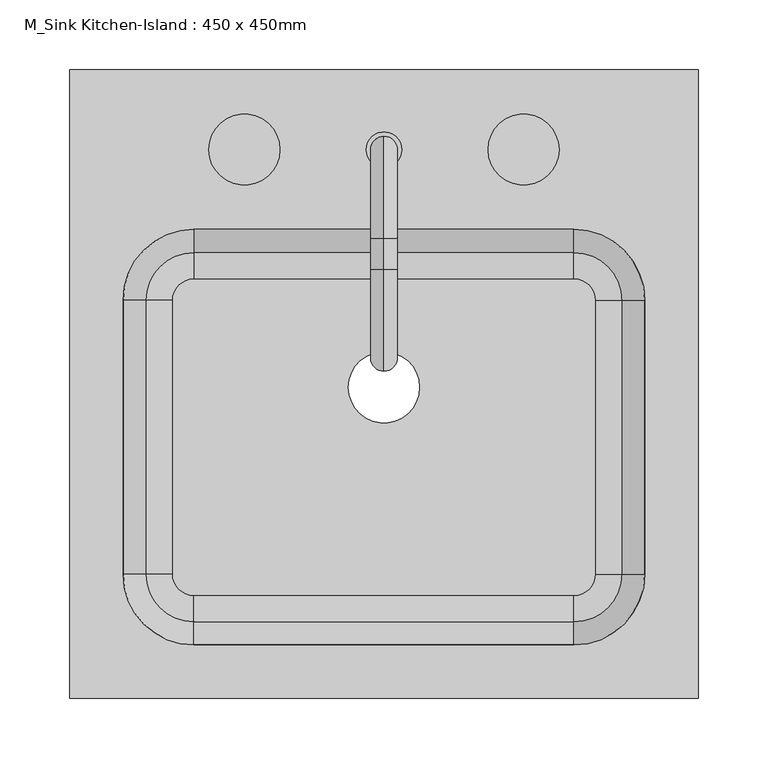
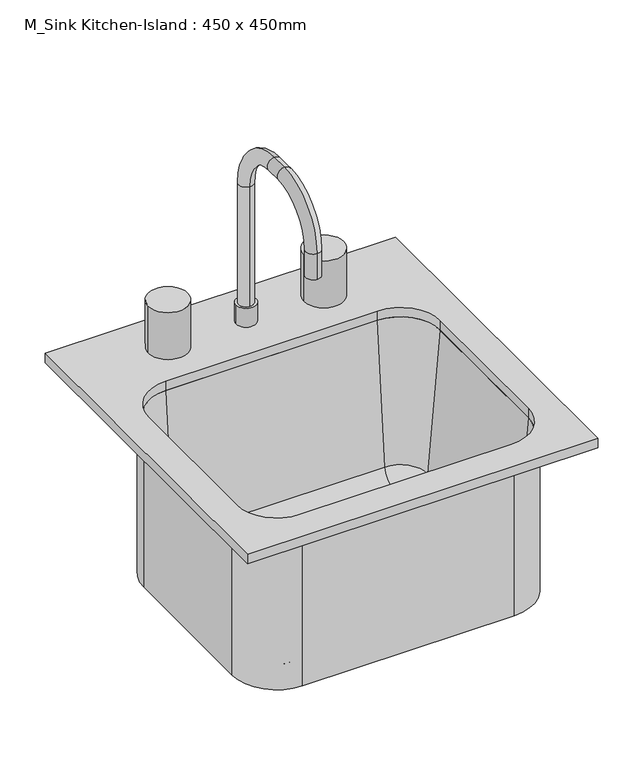
"""IFC4 building model written with IfcOpenShell, lengths in millimetres: flow terminal geometry, M_Sink Kitchen-Island : 450 x 450mm."""

from ifc_helpers import new_model, si_unit, point, frame, frame_2d, origin, place, context, project, spatial, polyline, circle_curve, ellipse_curve, trimmed, segment, composite_curve, outline, extrude, source, transform, mapped, element, save
from ifc_brep_helpers import plane_surface, cylinder_surface, revolved_surface, advanced_brep


def m_sink_kitchen_island_450_x_450mm_f969cf2d(model_context):
    return source(origin(), model_context, "Body", "SolidModel", [
        advanced_brep(
        [(208.9392406, 62.2454011, 684.1), (151.7892406, 119.3954011, 684.1), (151.7892406, 119.3954011, 900.0), (208.9392406, 62.2454011, 900.0), (208.9392406, -133.7545989, 684.1), (151.7892406, -190.9045989, 684.1), (-120.4107594, -190.9045989, 684.1), (-177.5607594, -133.7545989, 684.1), (-177.5607594, 62.2454011, 684.1), (-120.4107594, 119.3954011, 684.1), (-9.7107594, 0.0, 684.1), (41.0892406, 0.0, 684.1), (167.0776588, 62.2454011, 693.625), (151.7892406, 77.5338193, 693.625), (-120.4107594, 77.5338193, 693.625), (-135.6991776, 62.2454011, 693.625), (-135.6991776, -133.7545989, 693.625), (-120.4107594, -149.0430171, 693.625), (151.7892406, -149.0430171, 693.625), (167.0776588, -133.7545989, 693.625), (-9.7107594, 0.0, 693.625), (41.0892406, 0.0, 693.625), (186.0551678, 62.2454011, 711.0146831), (151.7892406, 96.5113283, 711.0146831), (202.5892406, 62.2454011, 900.0), (151.7892406, 113.0454011, 900.0), (208.9392406, -133.7545989, 900.0), (186.0551678, -133.7545989, 711.0146831), (202.5892406, -133.7545989, 900.0), (151.7892406, -190.9045989, 900.0), (151.7892406, -168.0205261, 711.0146831), (151.7892406, -184.5545989, 900.0), (-120.4107594, -190.9045989, 900.0), (-120.4107594, -168.0205261, 711.0146831), (-120.4107594, -184.5545989, 900.0), (-177.5607594, -133.7545989, 900.0), (-154.6766866, -133.7545989, 711.0146831), (-171.2107594, -133.7545989, 900.0), (-177.5607594, 62.2454011, 900.0), (-154.6766866, 62.2454011, 711.0146831), (-171.2107594, 62.2454011, 900.0), (-120.4107594, 119.3954011, 900.0), (-120.4107594, 96.5113283, 711.0146831), (-120.4107594, 113.0454011, 900.0)],
        [
            (0, 1, circle_curve(frame((151.7892406, 62.2454011, 684.1), z_axis=(0.0, 0.0, 1.0), x_axis=(0.0, 1.0, 0.0)), 57.15)),
            (1, 2),
            (2, 3, circle_curve(frame((151.7892406, 62.2454011, 900.0), z_axis=(0.0, 0.0, -1.0), x_axis=(0.0, 1.0, 0.0)), 57.15)),
            (3, 0),
            (0, 4),
            (4, 5, circle_curve(frame((151.7892406, -133.7545989, 684.1), z_axis=(0.0, 0.0, -1.0), x_axis=(1.0, 0.0, 0.0)), 57.15)),
            (5, 6),
            (6, 7, circle_curve(frame((-120.4107594, -133.7545989, 684.1), z_axis=(0.0, 0.0, -1.0), x_axis=(0.0, -1.0, 0.0)), 57.15)),
            (7, 8),
            (8, 9, circle_curve(frame((-120.4107594, 62.2454011, 684.1), z_axis=(0.0, 0.0, -1.0), x_axis=(-1.0, 0.0, 0.0)), 57.15)),
            (9, 1),
            (10, 11, circle_curve(frame((15.6892406, 0.0, 684.1), z_axis=(0.0, 0.0, 1.0), x_axis=(1.0, 0.0, 0.0)), 25.4)),
            (11, 10, circle_curve(frame((15.6892406, 0.0, 684.1), z_axis=(0.0, 0.0, 1.0), x_axis=(1.0, 0.0, 0.0)), 25.4)),
            (12, 13, circle_curve(frame((151.7892406, 62.2454011, 693.625), z_axis=(0.0, 0.0, 1.0), x_axis=(0.0, 1.0, 0.0)), 15.2884182)),
            (13, 14),
            (14, 15, circle_curve(frame((-120.4107594, 62.2454011, 693.625), z_axis=(0.0, 0.0, 1.0), x_axis=(-1.0, 0.0, 0.0)), 15.2884182)),
            (15, 16),
            (16, 17, circle_curve(frame((-120.4107594, -133.7545989, 693.625), z_axis=(0.0, 0.0, 1.0), x_axis=(0.0, -1.0, 0.0)), 15.2884182)),
            (17, 18),
            (18, 19, circle_curve(frame((151.7892406, -133.7545989, 693.625), z_axis=(0.0, 0.0, 1.0), x_axis=(1.0, 0.0, 0.0)), 15.2884182)),
            (19, 12),
            (20, 21, circle_curve(frame((15.6892406, 0.0, 693.625), z_axis=(0.0, 0.0, -1.0), x_axis=(1.0, 0.0, 0.0)), 25.4)),
            (21, 20, circle_curve(frame((15.6892406, 0.0, 693.625), z_axis=(0.0, 0.0, -1.0), x_axis=(1.0, 0.0, 0.0)), 25.4)),
            (12, 22, circle_curve(frame((167.0776588, 62.2454011, 712.675), z_axis=(0.0, -1.0, 0.0), x_axis=(1.0, 0.0, 0.0)), 19.05)),
            (22, 23, circle_curve(frame((151.7892406, 62.2454011, 711.0146831), z_axis=(0.0, 0.0, 1.0), x_axis=(0.0, 1.0, 0.0)), 34.2659272)),
            (23, 13, circle_curve(frame((151.7892406, 77.5338193, 712.675), z_axis=(-1.0, 0.0, 0.0), x_axis=(0.0, 1.0, 0.0)), 19.05)),
            (22, 24),
            (24, 25, circle_curve(frame((151.7892406, 62.2454011, 900.0), z_axis=(0.0, 0.0, 1.0), x_axis=(0.0, 1.0, 0.0)), 50.8)),
            (25, 23),
            (2, 25),
            (24, 3),
            (3, 26),
            (26, 4),
            (19, 27, circle_curve(frame((167.0776588, -133.7545989, 712.675), z_axis=(0.0, -1.0, 0.0), x_axis=(1.0, 0.0, 0.0)), 19.05)),
            (27, 22),
            (27, 28),
            (28, 24),
            (28, 26),
            (26, 29, circle_curve(frame((151.7892406, -133.7545989, 900.0), z_axis=(0.0, 0.0, -1.0), x_axis=(1.0, 0.0, 0.0)), 57.15)),
            (29, 5),
            (18, 30, circle_curve(frame((151.7892406, -149.0430171, 712.675), z_axis=(-1.0, 0.0, 0.0), x_axis=(0.0, -1.0, 0.0)), 19.05)),
            (30, 27, circle_curve(frame((151.7892406, -133.7545989, 711.0146831), z_axis=(0.0, 0.0, 1.0), x_axis=(1.0, 0.0, 0.0)), 34.2659272)),
            (30, 31),
            (31, 28, circle_curve(frame((151.7892406, -133.7545989, 900.0), z_axis=(0.0, 0.0, 1.0), x_axis=(1.0, 0.0, 0.0)), 50.8)),
            (31, 29),
            (29, 32),
            (32, 6),
            (17, 33, circle_curve(frame((-120.4107594, -149.0430171, 712.675), z_axis=(-1.0, 0.0, 0.0), x_axis=(0.0, -1.0, 0.0)), 19.05)),
            (33, 30),
            (33, 34),
            (34, 31),
            (34, 32),
            (32, 35, circle_curve(frame((-120.4107594, -133.7545989, 900.0), z_axis=(0.0, 0.0, -1.0), x_axis=(0.0, -1.0, 0.0)), 57.15)),
            (35, 7),
            (16, 36, circle_curve(frame((-135.6991776, -133.7545989, 712.675), z_axis=(0.0, 1.0, 0.0), x_axis=(-1.0, 0.0, 0.0)), 19.05)),
            (36, 33, circle_curve(frame((-120.4107594, -133.7545989, 711.0146831), z_axis=(0.0, 0.0, 1.0), x_axis=(0.0, -1.0, 0.0)), 34.2659272)),
            (36, 37),
            (37, 34, circle_curve(frame((-120.4107594, -133.7545989, 900.0), z_axis=(0.0, 0.0, 1.0), x_axis=(0.0, -1.0, 0.0)), 50.8)),
            (37, 35),
            (35, 38),
            (38, 8),
            (15, 39, circle_curve(frame((-135.6991776, 62.2454011, 712.675), z_axis=(0.0, 1.0, 0.0), x_axis=(-1.0, 0.0, 0.0)), 19.05)),
            (39, 36),
            (39, 40),
            (40, 37),
            (40, 38),
            (38, 41, circle_curve(frame((-120.4107594, 62.2454011, 900.0), z_axis=(0.0, 0.0, -1.0), x_axis=(-1.0, 0.0, 0.0)), 57.15)),
            (41, 9),
            (14, 42, circle_curve(frame((-120.4107594, 77.5338193, 712.675), z_axis=(1.0, 0.0, 0.0), x_axis=(0.0, 1.0, 0.0)), 19.05)),
            (42, 39, circle_curve(frame((-120.4107594, 62.2454011, 711.0146831), z_axis=(0.0, 0.0, 1.0), x_axis=(-1.0, 0.0, 0.0)), 34.2659272)),
            (42, 43),
            (43, 40, circle_curve(frame((-120.4107594, 62.2454011, 900.0), z_axis=(0.0, 0.0, 1.0), x_axis=(-1.0, 0.0, 0.0)), 50.8)),
            (43, 41),
            (41, 2),
            (23, 42),
            (25, 43),
            (20, 10),
            (11, 21),
        ],
        [
            cylinder_surface(frame((151.7892406, 62.2454011, 0.0), z_axis=(0.0, 0.0, -1.0), x_axis=(0.0, 1.0, 0.0)), 57.15),
            plane_surface(frame((151.7892406, 62.2454011, 684.1), z_axis=(0.0, 0.0, -1.0), x_axis=(0.0, 1.0, 0.0))),
            plane_surface(frame((151.7892406, 62.2454011, 693.625), z_axis=(0.0, 0.0, 1.0), x_axis=(0.0, 1.0, 0.0))),
            revolved_surface(trimmed(ellipse_curve(frame((151.7892406, 77.5338193, 712.675), z_axis=(1.0, 0.0, 0.0), x_axis=(0.0, 1.0, 0.0)), 19.05, 19.05), [point((151.7892406, 77.5338193, 693.625))], [point((151.7892406, 96.5113283, 711.0146831))], True, "CARTESIAN"), (151.7892406, 62.2454011, 0.0), (0.0, 0.0, -1.0)),
            revolved_surface(polyline([(151.7892406, 96.5113283, 711.0146831), (151.7892406, 113.0454011, 900.0)]), (151.7892406, 62.2454011, 0.0), (0.0, 0.0, -1.0)),
            plane_surface(frame((151.7892406, 62.2454011, 900.0), z_axis=(0.0, 0.0, 1.0), x_axis=(0.0, 1.0, 0.0))),
            plane_surface(frame((208.9392406, 62.2454011, 900.0), z_axis=(1.0, 0.0, 0.0), x_axis=(0.0, -1.0, 0.0))),
            revolved_surface(polyline([(186.1276588, -133.7545989, 712.675), (186.1276588, 62.2454011, 712.675)]), (167.0776588, 62.2454011, 712.675), (0.0, -1.0, 0.0)),
            plane_surface(frame((186.0551678, 62.2454011, 711.0146831), z_axis=(-0.9961946980917444, 0.0, 0.0871557427476718), x_axis=(0.0, -1.0, 0.0))),
            plane_surface(frame((202.5892406, 62.2454011, 900.0), z_axis=(0.0, 0.0, 1.0), x_axis=(0.0, -1.0, 0.0))),
            cylinder_surface(frame((151.7892406, -133.7545989, 0.0), z_axis=(0.0, 0.0, -1.0), x_axis=(1.0, 0.0, 0.0)), 57.15),
            revolved_surface(trimmed(ellipse_curve(frame((167.0776588, -133.7545989, 712.675), z_axis=(0.0, -1.0, 0.0), x_axis=(1.0, 0.0, 0.0)), 19.05, 19.05), [point((167.0776588, -133.7545989, 693.625))], [point((186.0551678, -133.7545989, 711.0146831))], True, "CARTESIAN"), (151.7892406, -133.7545989, 0.0), (0.0, 0.0, -1.0)),
            revolved_surface(polyline([(186.0551678, -133.7545989, 711.0146831), (202.5892406, -133.7545989, 900.0)]), (151.7892406, -133.7545989, 0.0), (0.0, 0.0, -1.0)),
            plane_surface(frame((151.7892406, -133.7545989, 900.0), z_axis=(0.0, 0.0, 1.0), x_axis=(1.0, 0.0, 0.0))),
            plane_surface(frame((151.7892406, -190.9045989, 900.0), z_axis=(0.0, -1.0, 0.0), x_axis=(-1.0, 0.0, 0.0))),
            revolved_surface(polyline([(-120.41075939999999, -168.0930171, 712.675), (151.7892406, -168.0930171, 712.675)]), (151.7892406, -149.0430171, 712.675), (-1.0, 0.0, 0.0)),
            plane_surface(frame((151.7892406, -168.0205261, 711.0146831), z_axis=(0.0, 0.9961946980917444, 0.0871557427476718), x_axis=(-1.0, 0.0, 0.0))),
            plane_surface(frame((151.7892406, -184.5545989, 900.0), z_axis=(0.0, 0.0, 1.0), x_axis=(-1.0, 0.0, 0.0))),
            cylinder_surface(frame((-120.4107594, -133.7545989, 0.0), z_axis=(0.0, 0.0, -1.0), x_axis=(0.0, -1.0, 0.0)), 57.15),
            revolved_surface(trimmed(ellipse_curve(frame((-120.4107594, -149.0430171, 712.675), z_axis=(-1.0, 0.0, 0.0), x_axis=(0.0, -1.0, 0.0)), 19.05, 19.05), [point((-120.4107594, -149.0430171, 693.625))], [point((-120.4107594, -168.0205261, 711.0146831))], True, "CARTESIAN"), (-120.4107594, -133.7545989, 0.0), (0.0, 0.0, -1.0)),
            revolved_surface(polyline([(-120.4107594, -168.0205261, 711.0146831), (-120.4107594, -184.5545989, 900.0)]), (-120.4107594, -133.7545989, 0.0), (0.0, 0.0, -1.0)),
            plane_surface(frame((-120.4107594, -133.7545989, 900.0), z_axis=(0.0, 0.0, 1.0), x_axis=(0.0, -1.0, 0.0))),
            plane_surface(frame((-177.5607594, -133.7545989, 900.0), z_axis=(-1.0, 0.0, 0.0), x_axis=(0.0, 1.0, 0.0))),
            revolved_surface(polyline([(-154.74917760000002, 62.24540110000001, 712.675), (-154.74917760000002, -133.7545989, 712.675)]), (-135.6991776, -133.7545989, 712.675), (0.0, 1.0, 0.0)),
            plane_surface(frame((-154.6766866, -133.7545989, 711.0146831), z_axis=(0.9961946980917444, 0.0, 0.0871557427476718), x_axis=(0.0, 1.0, 0.0))),
            plane_surface(frame((-171.2107594, -133.7545989, 900.0), z_axis=(0.0, 0.0, 1.0), x_axis=(0.0, 1.0, 0.0))),
            cylinder_surface(frame((-120.4107594, 62.2454011, 0.0), z_axis=(0.0, 0.0, -1.0), x_axis=(-1.0, 0.0, 0.0)), 57.15),
            revolved_surface(trimmed(ellipse_curve(frame((-135.6991776, 62.2454011, 712.675), z_axis=(0.0, 1.0, 0.0), x_axis=(-1.0, 0.0, 0.0)), 19.05, 19.05), [point((-135.6991776, 62.2454011, 693.625))], [point((-154.6766866, 62.2454011, 711.0146831))], True, "CARTESIAN"), (-120.4107594, 62.2454011, 0.0), (0.0, 0.0, -1.0)),
            revolved_surface(polyline([(-154.6766866, 62.2454011, 711.0146831), (-171.2107594, 62.2454011, 900.0)]), (-120.4107594, 62.2454011, 0.0), (0.0, 0.0, -1.0)),
            plane_surface(frame((-120.4107594, 62.2454011, 900.0), z_axis=(0.0, 0.0, 1.0), x_axis=(-1.0, 0.0, 0.0))),
            plane_surface(frame((-120.4107594, 119.3954011, 900.0), z_axis=(0.0, 1.0, 0.0), x_axis=(1.0, 0.0, 0.0))),
            revolved_surface(polyline([(151.78924059999997, 96.5838193, 712.675), (-120.4107594, 96.5838193, 712.675)]), (-120.4107594, 77.5338193, 712.675), (1.0, 0.0, 0.0)),
            plane_surface(frame((-120.4107594, 96.5113283, 711.0146831), z_axis=(0.0, -0.9961946980917444, 0.0871557427476718), x_axis=(1.0, 0.0, 0.0))),
            plane_surface(frame((-120.4107594, 113.0454011, 900.0), z_axis=(0.0, 0.0, 1.0), x_axis=(1.0, 0.0, 0.0))),
            revolved_surface(polyline([(41.0892406, 0.0, 684.1), (41.0892406, 0.0, 693.625)]), (15.6892406, 0.0, 0.0), (0.0, 0.0, -1.0)),
        ],
        [
            (0, [[1, 2, 3, 4]]),
            (1, [[-1, 5, 6, 7, 8, 9, 10, 11], [12, 13]]),
            (2, [[14, 15, 16, 17, 18, 19, 20, 21], [22, 23]]),
            (3, [[-14, 24, 25, 26]]),
            (4, [[-25, 27, 28, 29]]),
            (5, [[-3, 30, -28, 31]]),
            (6, [[-4, 32, 33, -5]]),
            (7, [[-24, -21, 34, 35]]),
            (8, [[-27, -35, 36, 37]]),
            (9, [[-31, -37, 38, -32]]),
            (10, [[-33, 39, 40, -6]]),
            (11, [[-34, -20, 41, 42]]),
            (12, [[-36, -42, 43, 44]]),
            (13, [[-38, -44, 45, -39]]),
            (14, [[-40, 46, 47, -7]]),
            (15, [[-41, -19, 48, 49]]),
            (16, [[-43, -49, 50, 51]]),
            (17, [[-45, -51, 52, -46]]),
            (18, [[-47, 53, 54, -8]]),
            (19, [[-48, -18, 55, 56]]),
            (20, [[-50, -56, 57, 58]]),
            (21, [[-52, -58, 59, -53]]),
            (22, [[-54, 60, 61, -9]]),
            (23, [[-55, -17, 62, 63]]),
            (24, [[-57, -63, 64, 65]]),
            (25, [[-59, -65, 66, -60]]),
            (26, [[-61, 67, 68, -10]]),
            (27, [[-62, -16, 69, 70]]),
            (28, [[-64, -70, 71, 72]]),
            (29, [[-66, -72, 73, -67]]),
            (30, [[-2, -11, -68, 74]]),
            (31, [[-26, 75, -69, -15]]),
            (32, [[-29, 76, -71, -75]]),
            (33, [[-30, -74, -73, -76]]),
            (34, [[-22, 77, -13, 78]]),
            (34, [[-23, -78, -12, -77]]),
        ],
    ),
        advanced_brep(
        [(2.9892406, 170.1954011, 912.7), (28.3892406, 170.1954011, 912.7), (15.6892406, 179.7204011, 1100.025), (15.6892406, 160.6704011, 1100.025), (15.6892406, 160.6704011, 938.1), (15.6892406, 179.7204011, 938.1), (15.6892406, 106.6954011, 1173.05), (15.6892406, 106.6954011, 1154.0), (15.6892406, 84.4704011, 1173.05), (15.6892406, 84.4704011, 1154.0), (15.6892406, 11.4454011, 1100.025), (15.6892406, 30.4954011, 1100.025), (15.6892406, 11.4454011, 1065.1), (15.6892406, 30.4954011, 1065.1), (2.9892406, 170.1954011, 938.1), (28.3892406, 170.1954011, 938.1)],
        [
            (0, 1, circle_curve(frame((15.6892406, 170.1954011, 912.7), z_axis=(0.0, 0.0, -1.0), x_axis=(1.0, 0.0, 0.0)), 12.7)),
            (1, 0, circle_curve(frame((15.6892406, 170.1954011, 912.7), z_axis=(0.0, 0.0, -1.0), x_axis=(1.0, 0.0, 0.0)), 12.7)),
            (2, 3, circle_curve(frame((15.6892406, 170.1954011, 1100.025), z_axis=(0.0, 0.0, -1.0), x_axis=(0.0, -1.0, 0.0)), 9.525)),
            (3, 4),
            (4, 5, circle_curve(frame((15.6892406, 170.1954011, 938.1), z_axis=(0.0, 0.0, 1.0), x_axis=(0.0, -1.0, 0.0)), 9.525)),
            (5, 2),
            (3, 2, circle_curve(frame((15.6892406, 170.1954011, 1100.025), z_axis=(0.0, 0.0, -1.0), x_axis=(0.0, -1.0, 0.0)), 9.525)),
            (5, 4, circle_curve(frame((15.6892406, 170.1954011, 938.1), z_axis=(0.0, 0.0, 1.0), x_axis=(0.0, -1.0, 0.0)), 9.525)),
            (2, 6, circle_curve(frame((15.6892406, 106.6954011, 1100.025), z_axis=(1.0, 0.0, 0.0), x_axis=(0.0, 1.0, 0.0)), 73.025)),
            (6, 7, circle_curve(frame((15.6892406, 106.6954011, 1163.525), z_axis=(0.0, 1.0, 0.0), x_axis=(0.0, 0.0, -1.0)), 9.525)),
            (7, 3, circle_curve(frame((15.6892406, 106.6954011, 1100.025), z_axis=(-1.0, 0.0, 0.0), x_axis=(0.0, 1.0, 0.0)), 53.975)),
            (7, 6, circle_curve(frame((15.6892406, 106.6954011, 1163.525), z_axis=(0.0, 1.0, 0.0), x_axis=(0.0, 0.0, -1.0)), 9.525)),
            (6, 8),
            (8, 9, circle_curve(frame((15.6892406, 84.4704011, 1163.525), z_axis=(0.0, 1.0, 0.0), x_axis=(0.0, 0.0, -1.0)), 9.525)),
            (9, 7),
            (9, 8, circle_curve(frame((15.6892406, 84.4704011, 1163.525), z_axis=(0.0, 1.0, 0.0), x_axis=(0.0, 0.0, -1.0)), 9.525)),
            (8, 10, circle_curve(frame((15.6892406, 84.4704011, 1100.025), z_axis=(1.0, 0.0, 0.0), x_axis=(0.0, 0.0, 1.0)), 73.025)),
            (10, 11, circle_curve(frame((15.6892406, 20.9704011, 1100.025), z_axis=(0.0, 0.0, 1.0), x_axis=(0.0, 1.0, 0.0)), 9.525)),
            (11, 9, circle_curve(frame((15.6892406, 84.4704011, 1100.025), z_axis=(-1.0, 0.0, 0.0), x_axis=(0.0, 0.0, 1.0)), 53.975)),
            (11, 10, circle_curve(frame((15.6892406, 20.9704011, 1100.025), z_axis=(0.0, 0.0, 1.0), x_axis=(0.0, 1.0, 0.0)), 9.525)),
            (12, 13, circle_curve(frame((15.6892406, 20.9704011, 1065.1), z_axis=(0.0, 0.0, -1.0), x_axis=(0.0, 1.0, 0.0)), 9.525)),
            (13, 12, circle_curve(frame((15.6892406, 20.9704011, 1065.1), z_axis=(0.0, 0.0, -1.0), x_axis=(0.0, 1.0, 0.0)), 9.525)),
            (10, 12),
            (13, 11),
            (14, 15, circle_curve(frame((15.6892406, 170.1954011, 938.1), z_axis=(0.0, 0.0, 1.0), x_axis=(1.0, 0.0, 0.0)), 12.7)),
            (15, 14, circle_curve(frame((15.6892406, 170.1954011, 938.1), z_axis=(0.0, 0.0, 1.0), x_axis=(1.0, 0.0, 0.0)), 12.7)),
            (14, 0),
            (1, 15),
        ],
        [
            plane_surface(frame((15.6892406, 160.6704011, 912.7), z_axis=(0.0, 0.0, -1.0), x_axis=(1.0, 0.0, 0.0))),
            cylinder_surface(frame((15.6892406, 170.1954011, 912.7), z_axis=(0.0, 0.0, -1.0), x_axis=(0.0, -1.0, 0.0)), 9.525),
            revolved_surface(trimmed(ellipse_curve(frame((15.6892406, 170.1954011, 1100.025), z_axis=(0.0, 0.0, -1.0), x_axis=(0.0, -1.0, 0.0)), 9.525, 9.525), [point((15.6892406, 179.7204011, 1100.025))], [point((15.6892406, 160.6704011, 1100.025))], True, "CARTESIAN"), (15.6892406, 106.6954011, 1100.025), (1.0, 0.0, 0.0)),
            revolved_surface(trimmed(ellipse_curve(frame((15.6892406, 170.1954011, 1100.025), z_axis=(0.0, 0.0, -1.0), x_axis=(0.0, -1.0, 0.0)), 9.525, 9.525), [point((15.6892406, 160.6704011, 1100.025))], [point((15.6892406, 179.7204011, 1100.025))], True, "CARTESIAN"), (15.6892406, 106.6954011, 1100.025), (1.0, 0.0, 0.0)),
            cylinder_surface(frame((15.6892406, 106.6954011, 1163.525), z_axis=(0.0, 1.0, 0.0), x_axis=(0.0, 0.0, -1.0)), 9.525),
            revolved_surface(trimmed(ellipse_curve(frame((15.6892406, 84.4704011, 1163.525), z_axis=(0.0, 1.0, 0.0), x_axis=(0.0, 0.0, -1.0)), 9.525, 9.525), [point((15.6892406, 84.4704011, 1173.05))], [point((15.6892406, 84.4704011, 1154.0))], True, "CARTESIAN"), (15.6892406, 84.4704011, 1100.025), (1.0, 0.0, 0.0)),
            revolved_surface(trimmed(ellipse_curve(frame((15.6892406, 84.4704011, 1163.525), z_axis=(0.0, 1.0, 0.0), x_axis=(0.0, 0.0, -1.0)), 9.525, 9.525), [point((15.6892406, 84.4704011, 1154.0))], [point((15.6892406, 84.4704011, 1173.05))], True, "CARTESIAN"), (15.6892406, 84.4704011, 1100.025), (1.0, 0.0, 0.0)),
            plane_surface(frame((15.6892406, 11.4454011, 1065.1), z_axis=(0.0, 0.0, -1.0), x_axis=(-1.0, 0.0, 0.0))),
            cylinder_surface(frame((15.6892406, 20.9704011, 1100.025), z_axis=(0.0, 0.0, 1.0), x_axis=(0.0, 1.0, 0.0)), 9.525),
            plane_surface(frame((28.3892406, 170.1954011, 938.1), z_axis=(0.0, 0.0, 1.0), x_axis=(0.0, 1.0, 0.0))),
            cylinder_surface(frame((15.6892406, 170.1954011, 912.7), z_axis=(0.0, 0.0, 1.0), x_axis=(1.0, 0.0, 0.0)), 12.7),
        ],
        [
            (0, [[1, 2]]),
            (1, [[3, 4, 5, 6]]),
            (1, [[7, -6, 8, -4]]),
            (2, [[-3, 9, 10, 11]]),
            (3, [[-7, -11, 12, -9]]),
            (4, [[-10, 13, 14, 15]]),
            (4, [[-12, -15, 16, -13]]),
            (5, [[-14, 17, 18, 19]]),
            (6, [[-16, -19, 20, -17]]),
            (7, [[21, 22]]),
            (8, [[-18, 23, -22, 24]]),
            (8, [[-20, -24, -21, -23]]),
            (9, [[25, 26], [-5, -8]]),
            (10, [[-25, 27, -2, 28]]),
            (10, [[-26, -28, -1, -27]]),
        ],
    ),
        extrude(outline(composite_curve([segment(trimmed(circle_curve(frame_2d((-84.3107594, 170.1954011)), 25.4), [point((-109.7107594, 170.1954011))], [point((-58.9107594, 170.1954011))], False, "CARTESIAN"), True, "CONTINUOUS"), segment(trimmed(circle_curve(frame_2d((-84.3107594, 170.1954011)), 25.4), [point((-58.9107594, 170.1954011))], [point((-109.7107594, 170.1954011))], False, "CARTESIAN"), True, "CONTINUOUS")], self_intersect=False)), frame((0.0, 0.0, 912.7), z_axis=(0.0, 0.0, 1.0), x_axis=(1.0, 0.0, 0.0)), (0.0, 0.0, 1.0), 63.5),
        extrude(outline(composite_curve([segment(trimmed(circle_curve(frame_2d((115.6892406, 170.1954011)), 25.4), [point((90.2892406, 170.1954011))], [point((141.0892406, 170.1954011))], False, "CARTESIAN"), True, "CONTINUOUS"), segment(trimmed(circle_curve(frame_2d((115.6892406, 170.1954011)), 25.4), [point((141.0892406, 170.1954011))], [point((90.2892406, 170.1954011))], False, "CARTESIAN"), True, "CONTINUOUS")], self_intersect=False)), frame((0.0, 0.0, 912.7), z_axis=(0.0, 0.0, 1.0), x_axis=(1.0, 0.0, 0.0)), (0.0, 0.0, 1.0), 63.5),
        extrude(outline(polyline([(240.6892406, 227.3454011), (240.6892406, -222.6545989), (-209.3107594, -222.6545989), (-209.3107594, 227.3454011), (240.6892406, 227.3454011)]), holes=[composite_curve([segment(polyline([(151.7892406, 113.0454011), (-120.4107594, 113.0454011)]), True, "CONTINUOUS"), segment(trimmed(circle_curve(frame_2d((-120.4107594, 62.2454011)), 50.8), [point((-120.4107594, 113.0454011))], [point((-171.2107594, 62.2454011))], True, "CARTESIAN"), True, "CONTINUOUS"), segment(polyline([(-171.2107594, 62.2454011), (-171.2107594, -133.7545989)]), True, "CONTINUOUS"), segment(trimmed(circle_curve(frame_2d((-120.4107594, -133.7545989)), 50.8), [point((-171.2107594, -133.7545989))], [point((-120.4107594, -184.5545989))], True, "CARTESIAN"), True, "CONTINUOUS"), segment(polyline([(-120.4107594, -184.5545989), (151.7892406, -184.5545989)]), True, "CONTINUOUS"), segment(trimmed(circle_curve(frame_2d((151.7892406, -133.7545989)), 50.8), [point((151.7892406, -184.5545989))], [point((202.5892406, -133.7545989))], True, "CARTESIAN"), True, "CONTINUOUS"), segment(polyline([(202.5892406, -133.7545989), (202.5892406, 62.2454011)]), True, "CONTINUOUS"), segment(trimmed(circle_curve(frame_2d((151.7892406, 62.2454011)), 50.8), [point((202.5892406, 62.2454011))], [point((151.7892406, 113.0454011))], True, "CARTESIAN"), True, "CONTINUOUS")], self_intersect=False)]), frame((0.0, 0.0, 900.0), z_axis=(0.0, 0.0, 1.0), x_axis=(1.0, 0.0, 0.0)), (0.0, 0.0, 1.0), 12.7),
    ])


if __name__ == "__main__":
    model = new_model("IFC4")
    model_context = context("Model", 3, world=origin())
    ifc_project = project(units=[si_unit("LENGTHUNIT", "METRE", prefix="MILLI")], contexts=[model_context])
    site = spatial("IfcSite", under=ifc_project)
    building = spatial("IfcBuilding", under=site)
    placement = place(None, origin())
    m_sink_kitchen_island_450_x_450mm_shape = m_sink_kitchen_island_450_x_450mm_f969cf2d(model_context)
    element("IfcFlowTerminal", 1, ObjectType="M_Sink Kitchen-Island : 450 x 450mm", at=placement, inside=building, context=model_context, shape_type="MappedRepresentation", body=[
        mapped(m_sink_kitchen_island_450_x_450mm_shape, transform((0.0, 0.0, 0.0), x_axis=(1.0, 0.0, 0.0), y_axis=(0.0, 1.0, 0.0), z_axis=(0.0, 0.0, 1.0))),
    ])
    save(model, "model.ifc")

# Revit data of these elements
# Type "M_Sink Kitchen-Island : 450 x 450mm"
#   Counter Height [instance default] = 900 mm
#   Depth = 450 mm
#   Width = 450 mm
#   Fixture Material = Steel, Polished
#   Sink Material = Steel, Polished
#   Default Elevation = 0
# Element 1 (IfcFlowTerminal, "M_Sink Kitchen-Island : 450 x 450mm")
#   Materials on its faces: "Steel, Polished"
# Materials
#   "Steel, Polished": class "Metal", colour RGB 57 57 57, transparency 0, Description = "Polished steel", Cost = 0
